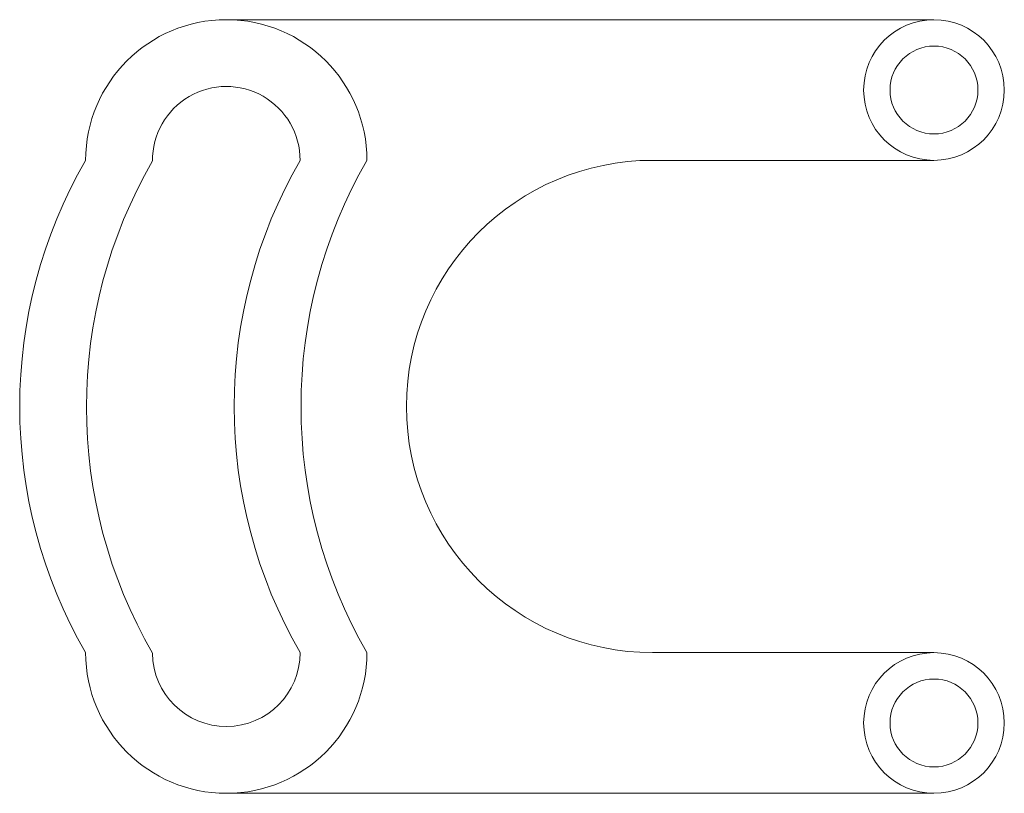
# Model space of a CAD drawing. Units: millimetres. Extents: x 5201 to 5341, y 655 to 765.
import ezdxf

# ---------------------------------------------------------------- set-up
doc = ezdxf.new("R2010")
doc.units = ezdxf.units.MM
doc.layers.add('M-CONS', color=8, linetype='Continuous', lineweight=18)

msp = doc.modelspace()

# ---------------------------------------------------------------- linework, layer by layer
at = {"layer": 'M-CONS'}
msp.add_line((5230.36, 654.99), (5330.98, 654.99), dxfattribs=at)
for points in [[(5210.36, 674.99, -0.267949), (5210.36, 744.99, -1), (5250.36, 744.99, 0.267949), (5250.36, 674.99, -1)], [(5219.86, 674.9, -0.267949), (5219.86, 744.9, -1.004358), (5240.86, 744.99, 0.267949), (5240.86, 674.99, -0.995661)]]:
    msp.add_lwpolyline(points, format="xyb", close=True, dxfattribs=at)
msp.add_lwpolyline([(5330.98, 764.99), (5230.36, 764.99)], dxfattribs=at)
msp.add_lwpolyline([(5330.98, 674.99), (5290.98, 674.99, -1), (5290.98, 744.99), (5330.98, 744.99)], format="xyb", dxfattribs=at)
for centre, radius in [((5330.98, 754.99), 10), ((5330.98, 754.99), 6.25), ((5330.98, 664.99), 10), ((5330.98, 664.99), 6.25)]:
    msp.add_circle(centre, radius, dxfattribs=at)
at = {"layer": 'M-CONS', "extrusion": (0, -1, 0)}
for radius in [12.5, 6.25]:
    msp.add_circle((5275.48, 46.07, -654.99), radius, dxfattribs=at)

doc.saveas('drawing.dxf')
